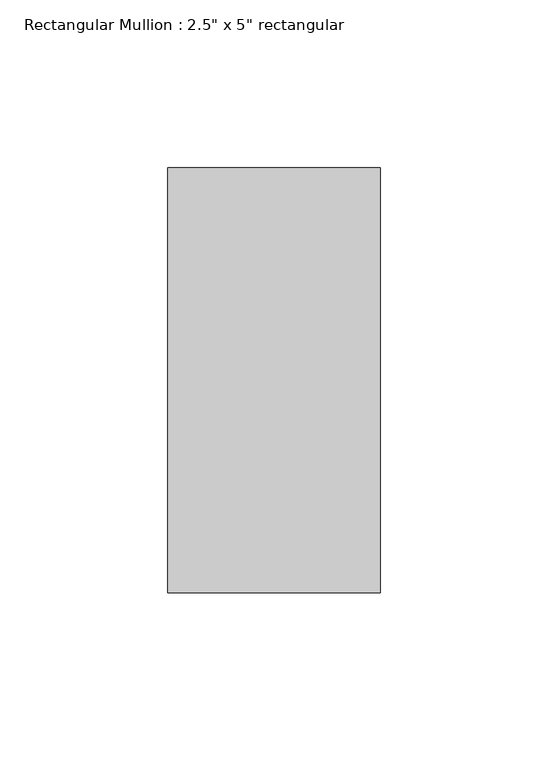
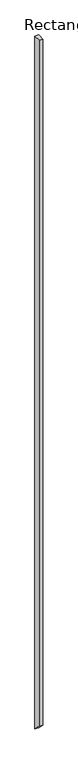
"""IFC4 building model written with IfcOpenShell, lengths in millimetres: member geometry."""

from ifc_helpers import new_model, si_unit, frame, origin, place, context, project, spatial, polyline, outline, extrude, source, transform, mapped, element, save


def member_fc190105(model_context):
    return source(origin(), model_context, "Body", "SweptSolid", [
        extrude(outline(polyline([(-63.5, 0.0), (63.5, 0.0), (63.5, -12885.7552746), (-63.5, -12758.7552746), (-63.5, 0.0)])), frame((-63.5, 0.0, 0.0), z_axis=(1.0, 0.0, 0.0), x_axis=(0.0, 1.0, 0.0)), (0.0, 0.0, 1.0), 63.5),
    ])


if __name__ == "__main__":
    model = new_model("IFC4")
    model_context = context("Model", 3, world=origin())
    ifc_project = project(units=[si_unit("LENGTHUNIT", "METRE", prefix="MILLI")], contexts=[model_context])
    site = spatial("IfcSite", under=ifc_project)
    building = spatial("IfcBuilding", under=site)
    placement = place(None, origin())
    member_shape = member_fc190105(model_context)
    element("IfcMember", 1, ObjectType="Rectangular Mullion : 2.5\" x 5\" rectangular", at=placement, inside=building, context=model_context, shape_type="MappedRepresentation", body=[
        mapped(member_shape, transform((0.0, 0.0, 0.0), x_axis=(1.0, 0.0, 0.0), y_axis=(0.0, 1.0, 0.0), z_axis=(0.0, 0.0, 1.0))),
    ])
    save(model, "model.ifc")

# Revit data of these elements
# Type "Rectangular Mullion : 2.5\" x 5\" rectangular"
#   built-in parameter 1007304 = 0.416667 (stored number, unit not read)
#   built-in parameter 1007301 = 0.104167 (stored number, unit not read)
#   built-in parameter 1007300 = 0.104167 (stored number, unit not read)
# Element 1 (IfcMember, "Rectangular Mullion : 2.5\" x 5\" rectangular")
#   Materials on its faces: "Aluminum"
# Materials
#   "Aluminum": class "Metal", colour RGB 247 247 247, transparency 0, Description = "Aluminum 6061", Cost = 0
